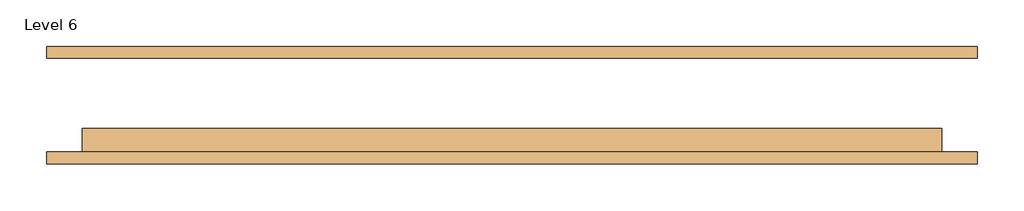
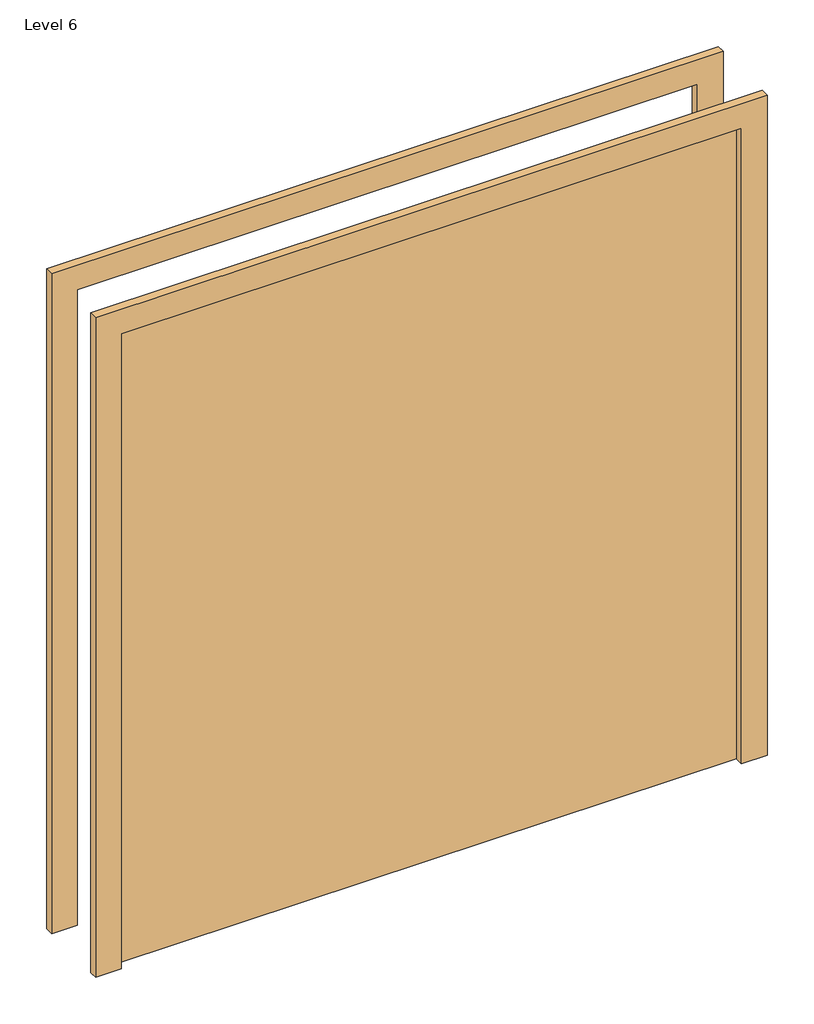
# One storey: 1 door.
"""IFC4 building model written with IfcOpenShell, lengths in millimetres."""

from ifc_helpers import new_model, si_unit, origin, place, context, project, spatial, transform, mapped, element, save
from components import door_8409b21c

model = new_model("IFC4")

# Units and contexts
model_context = context("Model", 3, world=origin())
ifc_project = project(units=[si_unit("LENGTHUNIT", "METRE", prefix="MILLI")], contexts=[model_context])

# Site, building, storey
site = spatial("IfcSite", under=ifc_project)
building = spatial("IfcBuilding", under=site)
storey = spatial("IfcBuildingStorey", under=building, Name="Level 6", Elevation=10096.0)

# Door
placement = place(None, origin())
door_shape = door_8409b21c(model_context)
element("IfcDoor", 1, ObjectType="Door-Double-Flush_Panel-Double-Acting : 72\" x 78\"", at=placement, inside=storey, context=model_context, shape_type="MappedRepresentation", body=[
    mapped(door_shape, transform((3177.920453, 2888.3992031, 8048.0), x_axis=(-1.0, 0.0, 0.0), y_axis=(0.0, -1.0, 0.0), z_axis=(0.0, 0.0, 1.0))),
])

save(model, "model.ifc")

# Revit data of these elements
# Type "Door-Double-Flush_Panel-Double-Acting : 72\" x 78\""
#   Type Mark = "22"
#   Construction Type Id = "DOOR"
#   Assembly Code = "C1020"
#   Analytic Construction = "Wooden"
#   W = 3' - 0"
#   Thickness = 0' - 2"
#   Thermal Resistance (R) = 0.455703 (m²·K)/W
#   Swing Angle [instance default] = 90.00°
#   Heat Transfer Coefficient (U) = 2.19465 W/(m²·K)
#   Height = 6' - 6"
#   Trim Projection Ext. = 0' - 1"
#   Trim Projection Int. = 0' - 1"
#   Trim Width Ext. = 0' - 3"
#   Trim Width Int. = 0' - 3"
#   Width = 6' - 0"
#   Define Thermal Properties by = 1
#   Panel Material = Wood - Birch - Solid Stained Light Low Gloss
#   Trim Material = Paint - Sienna
#   Visual Light Transmittance = 0
#   Solar Heat Gain Coefficient = 0
#   Function = (empty or 0)
#   Wall Closure = (empty or 0)
# Element 1 (IfcDoor, "Door-Double-Flush_Panel-Double-Acting : 72\" x 78\"")
#   Swing Angle = 90.00°
#   Phase Created = New Construction
#   Materials on its faces: "Paint - Sienna", "Wood - Birch - Solid Stained Light Low Gloss"
# Materials
#   "Wood - Birch - Solid Stained Light Low Gloss": class "Wood", colour RGB 210 159 95, transparency 0, Cost = 0
#   "Paint - Sienna": colour RGB 118 70 51, transparency 0, Cost = 0
